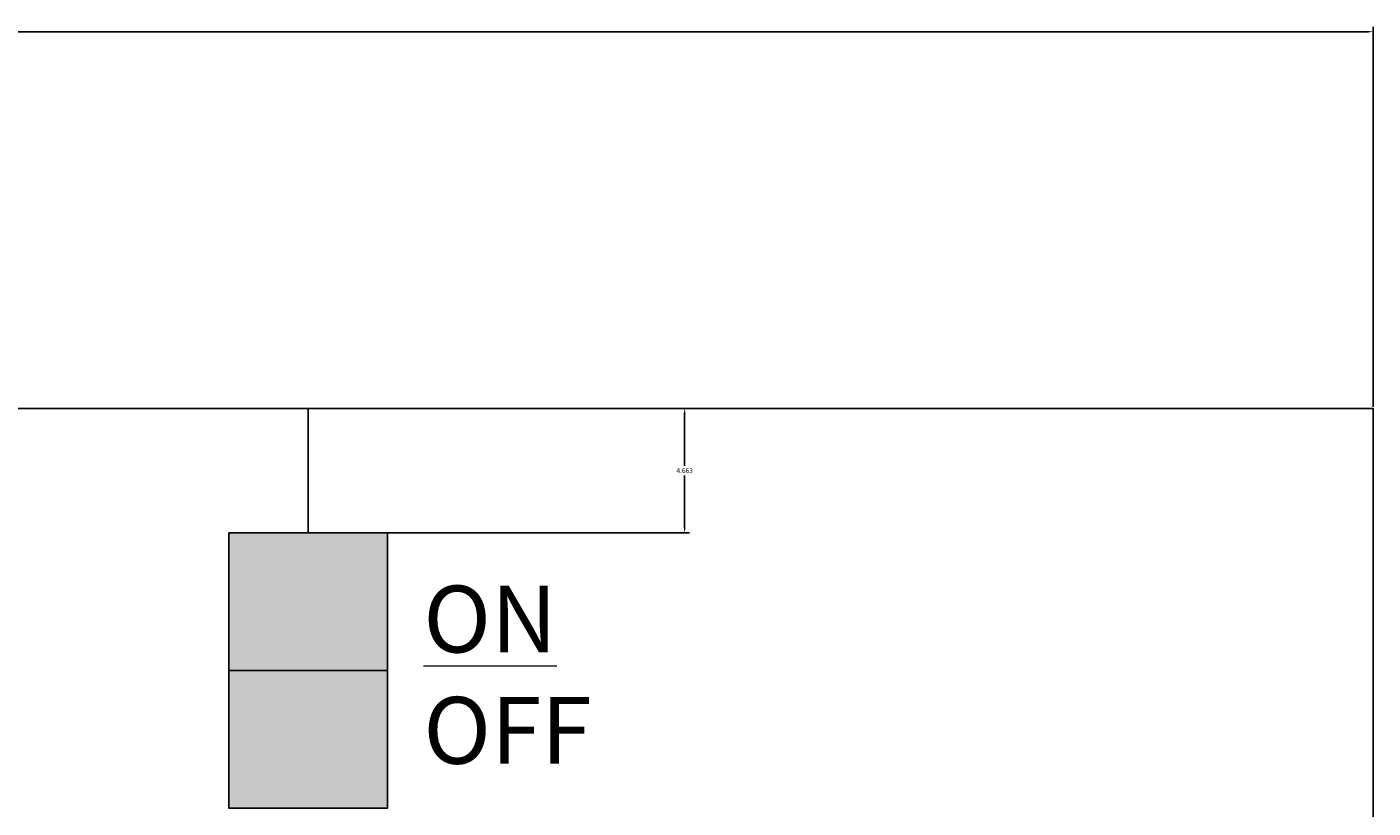
# Model space of a CAD drawing. Units: millimetres. Extents: x -8 to 285, y 5 to 221.
# Tile 30 of 30: x 221 to 271, y 191 to 221. Entities that reach past the tile are written whole.
import ezdxf

# ---------------------------------------------------------------- set-up
doc = ezdxf.new("R2010")
doc.units = ezdxf.units.MM
for name, color, linetype, lineweight in [('A-ANNO-DIMS', 2, 'Continuous', 18), ('E-ANNO-TEXT', 7, 'Continuous', 18), ('E-EQPM-PATT', 252, 'Continuous', 13), ('E-LITE-SWCH', 7, 'Continuous', 25)]:
    doc.layers.add(name, color=color, linetype=linetype, lineweight=lineweight)
doc.layers.add('E-POWR-AC-LINE', color=30, linetype='Continuous', lineweight=25, true_color=0xf26722)
doc.styles.get("Standard").update_dxf_attribs({"font": 'arial.ttf'})
doc.dimstyles.get("Standard").update_dxf_attribs({"dimtxt": 0.18, "dimasz": 0.18, "dimexe": 0.18, "dimexo": 0.0625, "dimgap": 0.09, "dimtad": 0, "dimtih": 1, "dimtoh": 1, "dimdec": 4, "dimzin": 0, "dimdsep": 46, "dimtxsty": 'Standard', "dimcen": 0.09, "dimadec": 0, "dimazin": 0, "dimtfac": 1, "dimtdec": 4, "dimtofl": 0, "dimtmove": 0, "dimatfit": 3, "dimfxl": 1, "dimtolj": 1, "dimtzin": 0, "dimarcsym": 0})

# ---------------------------------------------------------------- blocks, each defined once
blk = doc.blocks.new('SWITCH-ON-OFF')
blk.add_line((0, 5.151), (5.948, 5.151))
blk.add_lwpolyline([(0, 10.303), (5.948, 10.303), (5.948, 0), (0, 0)], close=True)
blk = doc.blocks.new('*D9')
at = {"layer": 'A-ANNO-DIMS', "color": 0, "lineweight": -2, "transparency": 16777216}
for p, q in [((6.672, 133.79), (6.672, 220.737)), ((6.852, 220.557), (138.33, 220.557)), ((270.739, 220.557), (139.262, 220.557)), ((270.919, 206.519), (270.919, 220.737))]:
    blk.add_line(p, q, dxfattribs=at)
at = {"layer": 'A-ANNO-DIMS', "color": 0, "transparency": 16777216}
for points in [[(6.852, 220.587), (6.852, 220.527), (6.672, 220.557)], [(270.739, 220.587), (270.739, 220.527), (270.919, 220.557)]]:
    blk.add_solid(points, dxfattribs=at)
at = {"layer": 'Defpoints', "color": 0, "transparency": 16777216}
for p in [(270.919, 220.557), (270.919, 206.457), (6.672, 133.727)]:
    blk.add_point(p, dxfattribs=at)
at = {"layer": 'A-ANNO-DIMS', "color": 0, "transparency": 16777216, "insert": (138.796, 220.557), "char_height": 0.18, "attachment_point": 5}
blk.add_mtext('\\A1;264.25', dxfattribs=at)
blk = doc.blocks.new('*D15')
at = {"layer": 'A-ANNO-DIMS', "color": 0, "lineweight": -2, "transparency": 16777216}
for p, q in [((231.104, 206.457), (245.321, 206.457)), ((245.141, 206.277), (245.141, 204.307)), ((245.141, 201.974), (245.141, 203.943)), ((231.104, 201.794), (245.321, 201.794))]:
    blk.add_line(p, q, dxfattribs=at)
at = {"layer": 'A-ANNO-DIMS', "color": 0, "transparency": 16777216}
for points in [[(245.111, 206.277), (245.171, 206.277), (245.141, 206.457)], [(245.111, 201.974), (245.171, 201.974), (245.141, 201.794)]]:
    blk.add_solid(points, dxfattribs=at)
at = {"layer": 'Defpoints', "color": 0, "transparency": 16777216}
for p in [(231.041, 206.457), (231.041, 201.794), (245.141, 201.794)]:
    blk.add_point(p, dxfattribs=at)
at = {"layer": 'A-ANNO-DIMS', "color": 0, "transparency": 16777216, "insert": (245.141, 204.125), "char_height": 0.18, "attachment_point": 5}
blk.add_mtext('\\A1;4.663', dxfattribs=at)

msp = doc.modelspace()

# ---------------------------------------------------------------- hatches: boundary and pattern name
at = {"layer": 'E-EQPM-PATT'}
h = msp.add_hatch(color=256, dxfattribs=at)
h.set_gradient(color2=(0, 0, 0), tint=1)
h.paths.add_polyline_path([(41.1717, 67.9064, 1), (39.1717, 67.9064, 1)])
h.paths.add_polyline_path([(47.1717, 67.9064, 1), (45.1717, 67.9064, 1)])
h.paths.add_polyline_path([(53.1717, 67.9064, 1), (51.1717, 67.9064, 1)])
h.paths.add_polyline_path([(57.1717, 67.9064, 1), (59.1717, 67.9064, 1)])
h.paths.add_polyline_path([(65.1717, 67.9064, 1), (63.1717, 67.9064, 1)])
h.paths.add_polyline_path([(69.1717, 67.9064, 1), (71.1717, 67.9064, 1)])
h.paths.add_polyline_path([(148.1394, 196.6424), (148.1394, 201.7939), (142.1909, 201.7939), (142.1909, 196.6424)])
h.paths.add_polyline_path([(186.1388, 201.7939), (186.1388, 196.6424), (192.0873, 196.6424), (192.0873, 201.7939)])
h.paths.add_polyline_path([(234.0155, 196.6424), (234.0155, 201.7939), (228.067, 201.7939), (228.067, 196.6424)])
h = msp.add_hatch(color=256, dxfattribs=at)
h.set_gradient(color1=(254, 234, 185), color2=(254, 234, 185), tint=1)
h.paths.add_polyline_path([(148.1394, 191.4908), (148.1394, 196.6424), (142.1909, 196.6424), (142.1909, 191.4908)])
h.paths.add_polyline_path([(186.1388, 191.4908), (192.0873, 191.4908), (192.0873, 196.6424), (186.1388, 196.6424)])
h.paths.add_polyline_path([(228.067, 191.4908), (234.0155, 191.4908), (234.0155, 196.6424), (228.067, 196.6424)])

# ---------------------------------------------------------------- linework, layer by layer
at = {"layer": 'E-POWR-AC-LINE'}
msp.add_line((231.0413, 201.7939), (231.0413, 206.4568), dxfattribs=at)
msp.add_lwpolyline([(244.6186, 34.6512), (244.6186, 49.925), (270.9192, 49.925), (270.9192, 206.4568), (145.1651, 206.4568), (145.1651, 201.7939)], dxfattribs=at)

# ---------------------------------------------------------------- block references
at = {"layer": 'E-LITE-SWCH'}
msp.add_blockref('SWITCH-ON-OFF', (228.0671, 191.491), dxfattribs=at)

# ---------------------------------------------------------------- texts
at = {"layer": 'E-ANNO-TEXT', "insert": (234.595, 199.8179), "char_height": 2.5, "attachment_point": 1}
msp.add_mtext_dynamic_manual_height_columns(' {\\LON\\P} OFF', width=8.619646, gutter_width=12.5, heights=[7.2553], dxfattribs=at)

# ---------------------------------------------------------------- dimensions: what is measured, and where the dimension line sits
at = {"layer": 'A-ANNO-DIMS'}
dim = msp.add_linear_dim(base=(270.9192, 220.5568), p1=(6.6725, 133.7273), p2=(270.9192, 206.4568), dimstyle='Standard', override={"dimdec": 2, "dimlfac": 1, "dimrnd": 0, "dimzin": 0, "dimdsep": 46, "dimlunit": 2}, dxfattribs=at)
dim.commit()
dim.dimension.update_dxf_attribs({"geometry": '*D9', "text_midpoint": (138.7958, 220.5568)})
dim = msp.add_linear_dim(base=(245.1413, 201.7939), p1=(231.0413, 206.4568), p2=(231.0413, 201.7939), angle=270, dimstyle='Standard', override={"dimdec": 3, "dimlfac": 1, "dimrnd": 0, "dimzin": 0, "dimdsep": 46, "dimlunit": 2}, dxfattribs=at)
dim.commit()
dim.dimension.update_dxf_attribs({"geometry": '*D15', "text_midpoint": (245.1413, 204.1254)})

doc.saveas('drawing.dxf')
